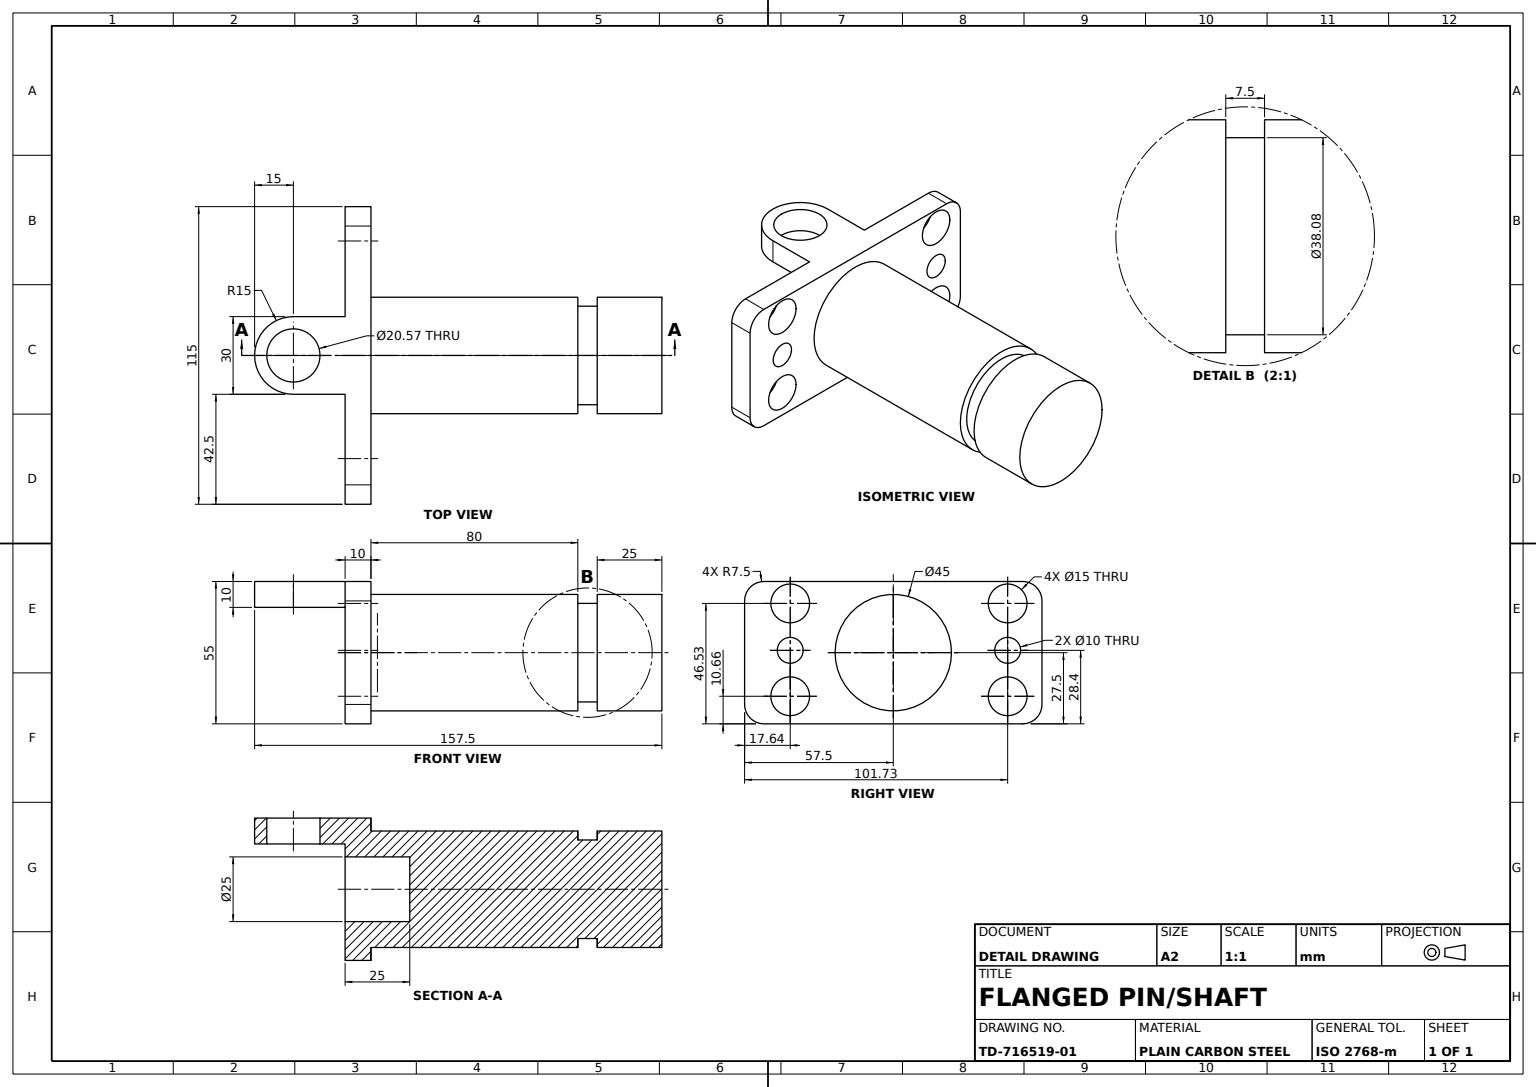
from build123d import *

# Parameters (mm, degrees)
FLANGE_PLATE_DEPTH      = 10
SHAFT_45_SKETCH_R       = 22.5
SHAFT_45_DEPTH          = 80
GROOVE_NECK_SKETCH_R    = 19.038570364
GROOVE_NECK_38_DEPTH    = 7.5
SHAFT_END_SKETCH_R      = 22.5
SHAFT_END_45_DEPTH      = 25
CENTRE_BORE_SKETCH_R    = 12.5
CENTRE_BORE_25_DEPTH    = 25
FLANGE_HOLES_SKETCH_R   = 7.5
FLANGE_HOLES_SKETCH_R_2 = 5
FLANGE_HOLES_6X_DEPTH   = 25
LUG_DEPTH               = 10
LUG_HOLE_SKETCH_R       = 10.286699657
LUG_HOLE_20_6_DEPTH     = 10


with BuildPart() as part:
    # Flange Plate Sketch → Flange Plate (new body)
    with BuildSketch(Plane.XY):
        with BuildLine():
            Line((0, 0), (50, 0))
            ThreePointArc((50, 0), (55.303300859, 2.196699141), (57.5, 7.5))
            Line((57.5, 7.5), (57.5, 47.5))
            ThreePointArc((57.5, 47.5), (55.303300859, 52.803300859), (50, 55))
            Line((50, 55), (-50, 55))
            ThreePointArc((-50, 55), (-55.303300859, 52.803300859), (-57.5, 47.5))
            Line((-57.5, 47.5), (-57.5, 7.5))
            ThreePointArc((-57.5, 7.5), (-55.303300859, 2.196699141), (-50, 0))
            Line((-50, 0), (0, 0))
        make_face()
    extrude(amount=FLANGE_PLATE_DEPTH)

    # Shaft Ø45 Sketch → Shaft Ø45 (add)
    with BuildSketch(Plane(origin=(0, 0, 0), x_dir=(-1, 0, 0), z_dir=(0, 0, -1))):
        with Locations((0, 27.5)):
            Circle(SHAFT_45_SKETCH_R)
    extrude(amount=SHAFT_45_DEPTH)

    # Groove Neck Sketch → Groove Neck Ø38 (add)
    with BuildSketch(Plane(origin=(0, 0, -80), x_dir=(-1, 0, 0), z_dir=(0, 0, -1))):
        with Locations((0, 27.5)):
            Circle(GROOVE_NECK_SKETCH_R)
    extrude(amount=GROOVE_NECK_38_DEPTH)

    # Shaft End Sketch → Shaft End Ø45 (add)
    with BuildSketch(Plane(origin=(0, 0, -87.5), x_dir=(-1, 0, 0), z_dir=(0, 0, -1))):
        with Locations((0, 27.5)):
            Circle(SHAFT_END_SKETCH_R)
    extrude(amount=SHAFT_END_45_DEPTH)

    # Centre Bore Sketch → Centre Bore Ø25 (cut)
    with BuildSketch(Plane.XY.offset(10)):
        with Locations((0, 27.5)):
            Circle(CENTRE_BORE_SKETCH_R)
    extrude(amount=-CENTRE_BORE_25_DEPTH, mode=Mode.SUBTRACT)

    # Flange Holes Sketch → Flange Holes 6x (cut)
    with BuildSketch(Plane.XY.offset(10)):
        with Locations((39.858984169, 46.529450506)):
            Circle(FLANGE_HOLES_SKETCH_R)
        with Locations((39.858984169, 28.400041578)):
            Circle(FLANGE_HOLES_SKETCH_R_2)
        with Locations((39.858984169, 10.656364754)):
            Circle(FLANGE_HOLES_SKETCH_R)
        with Locations((-44.230614691, 10.656364754)):
            Circle(FLANGE_HOLES_SKETCH_R)
        with Locations((-44.230614691, 28.400041578)):
            Circle(FLANGE_HOLES_SKETCH_R_2)
        with Locations((-44.230614691, 46.529450506)):
            Circle(FLANGE_HOLES_SKETCH_R)
    extrude(amount=-FLANGE_HOLES_6X_DEPTH, mode=Mode.SUBTRACT)

    # Lug Sketch → Lug (add)
    with BuildSketch(Plane(origin=(0, 55, 0), x_dir=(1, 0, 0), z_dir=(0, 1, 0))):
        with BuildLine():
            Line((0, -10), (-15, -10))
            Line((-15, -10), (-15, -30))
            ThreePointArc((-15, -30), (0, -45), (15, -30))
            Line((15, -30), (15, -10))
            Line((15, -10), (0, -10))
        make_face()
    extrude(amount=-LUG_DEPTH)

    # Lug Hole Sketch → Lug Hole Ø20.6 (cut)
    with BuildSketch(Plane.XZ.offset(-45)):
        with Locations(Location((0, 30, 0), (0, 0, 270))):
            Circle(LUG_HOLE_SKETCH_R)
    extrude(amount=-LUG_HOLE_20_6_DEPTH, mode=Mode.SUBTRACT)


solid = part.part
